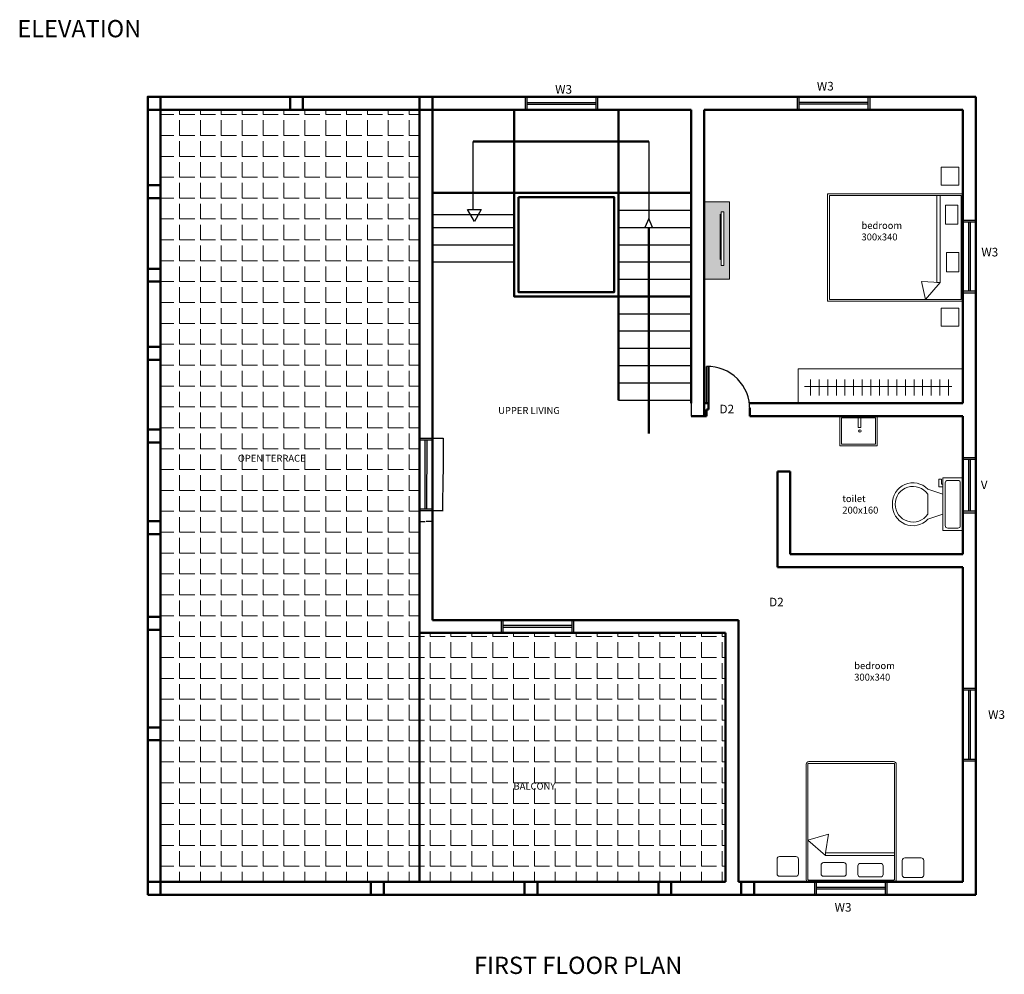
# Model space of a CAD drawing. Units: metres. Extents: x 10365 to 12529, y 3661 to 6248.
# Tile 2 of 9: x 11388 to 12529, y 3687 to 4794. Entities that reach past the tile are written whole.
import ezdxf

# ---------------------------------------------------------------- set-up
doc = ezdxf.new("R2010")
doc.units = ezdxf.units.M
doc.header["$MEASUREMENT"] = 0
for name, color, linetype, lineweight in [('A-ANNO-DIMS', 2, 'Continuous', 18), ('A-ANNO-TEXT', 7, 'Continuous', 18), ('A-AREA-IDEN', 7, 'Continuous', 18), ('A-DOOR', 4, 'Continuous', 25), ('A-FLOR-FIXT', 8, 'Continuous', 18), ('A-FLOR-PATT', 252, 'Continuous', 13), ('A-FLOR-STRS', 3, 'Continuous', 25), ('A-FURN', 30, 'Continuous', 18), ('A-GLAZ', 4, 'Continuous', 25), ('A-WALL', 7, 'Continuous', 50)]:
    doc.layers.add(name, color=color, linetype=linetype, lineweight=lineweight)
doc.styles.get("Standard").update_dxf_attribs({"font": 'arial.ttf'})
doc.dimstyles.get("Standard").update_dxf_attribs({"dimtxt": 0.18, "dimasz": 0.18, "dimexe": 0.18, "dimexo": 0.0625, "dimgap": 0.09, "dimtad": 0, "dimtih": 1, "dimtoh": 1, "dimdec": 0, "dimzin": 0, "dimdsep": 46, "dimtxsty": 'Standard', "dimcen": 0.09, "dimadec": 0, "dimazin": 0, "dimtfac": 1, "dimtdec": 0, "dimtofl": 0, "dimtmove": 0, "dimatfit": 3, "dimfxl": 1, "dimtolj": 1, "dimtzin": 0, "dimarcsym": 0})

# ---------------------------------------------------------------- blocks, each defined once
blk = doc.blocks.new('*U2')
for p, q in [((9.5, -6), (9.5, -2)), ((-10, -8.5), (-8, -8.5)), ((-10, -9.5), (-10, -8.5)), ((-7, -9.5), (-10, -9.5)), ((-8, -8.5), (-8, -8)), ((-7, -8), (-7, -9.5)), ((-4, -8), (-6, -14)), ((4, -8), (6, -14)), ((4, -14), (-4, -14))]:
    blk.add_line(p, q)
blk.add_lwpolyline([(10.5, -8), (10.5, 0), (-10.5, 0), (-10.5, -8)], close=True)
for points in [[(-9.5, -2), (-9.5, -6)], [(8.5, -1), (-8.5, -1)], [(-8.5, -7), (8.5, -7)]]:
    blk.add_lwpolyline(points)
for centre, radius, start, end in [((-8.625, -1.875), 0.8839, 81.8699, 188.1301), ((8.625, -1.875), 0.8839, 351.8699, 98.1301), ((-8.625, -6.125), 0.8839, 171.869898, 278.1301), ((8.625, -6.125), 0.8839, 261.8699, 8.1301), ((-0.4772, -19.9188), 8.0953, 133.01722, 273.38), ((0.0374, -19.8731), 7.127, 124.50543, 269.7), ((-0.0373, -19.8731), 7.127, 270.3, 55.4946), ((0.4773, -19.9188), 8.0953, 266.62, 46.9828)]:
    blk.add_arc(centre, radius, start, end)
blk = doc.blocks.new('DOOR-D2')
blk.add_line((0, 7.5), (0, 50))
blk.add_arc((1, 1), 49, 358.8309, 91.1691)
blk = doc.blocks.new('WIN-800')
for p, q in [((0, 0), (0, 15)), ((2, 0), (2, 15)), ((82, 0), (82, 15)), ((84, 0), (84, 15)), ((2, 8.5), (82, 8.5)), ((2, 6.5), (82, 6.5))]:
    blk.add_line(p, q)
blk = doc.blocks.new('VENT-600')
for p, q in [((0, 64), (15, 64)), ((0, 62), (15, 62)), ((6.5, 62), (6.5, 2)), ((8.5, 62), (8.5, 2)), ((8.5, 62), (8.5, 2)), ((0, 2), (15, 2)), ((0, 0), (15, 0))]:
    blk.add_line(p, q)
blk = doc.blocks.new('WIN-800-B')
for p, q in [((0, 84), (15, 84)), ((0, 82), (15, 82)), ((6.5, 82), (6.5, 2)), ((8.5, 82), (8.5, 2)), ((8.5, 82), (8.5, 2)), ((0, 2), (15, 2)), ((0, 0), (15, 0))]:
    blk.add_line(p, q)
blk = doc.blocks.new('*D19')
at = {"layer": 'A-ANNO-DIMS', "color": 0, "lineweight": -2, "transparency": 16777216}
for p, q in [((11866, 4308.7), (11878.7, 4308.6)), ((11878.6, 4308.4), (11878.4, 4266.8)), ((11878.3, 4224.8), (11878.4, 4266.4)), ((11865.7, 4224.7), (11878.5, 4224.6))]:
    blk.add_line(p, q, dxfattribs=at)
at = {"layer": 'A-ANNO-DIMS', "color": 0, "transparency": 16777216}
for points in [[(11878.5, 4308.4), (11878.6, 4308.4), (11878.6, 4308.6)], [(11878.3, 4224.8), (11878.3, 4224.8), (11878.3, 4224.6)]]:
    blk.add_solid(points, dxfattribs=at)
at = {"layer": 'Defpoints', "color": 0, "transparency": 16777216}
for p in [(11866, 4308.7), (11878.6, 4308.6), (11865.7, 4224.7)]:
    blk.add_point(p, dxfattribs=at)
at = {"layer": 'A-ANNO-DIMS', "color": 0, "transparency": 16777216, "insert": (11878.4, 4266.6), "char_height": 0.18, "attachment_point": 5}
blk.add_mtext('\\A1;WINDOW W3 84 TYP.', dxfattribs=at)
blk = doc.blocks.new('*D20')
at = {"layer": 'A-ANNO-DIMS', "color": 0, "lineweight": -2, "transparency": 16777216}
for p, q in [((11850.7, 4224.6), (11850.6, 4211.9)), ((11865.7, 4224.6), (11865.6, 4211.9)), ((11850.8, 4212.1), (11857.6, 4212.1)), ((11865.5, 4212.1), (11858.7, 4212.1))]:
    blk.add_line(p, q, dxfattribs=at)
at = {"layer": 'A-ANNO-DIMS', "color": 0, "transparency": 16777216}
for points in [[(11850.8, 4212.1), (11850.8, 4212.1), (11850.6, 4212.1)], [(11865.5, 4212.1), (11865.5, 4212), (11865.6, 4212.1)]]:
    blk.add_solid(points, dxfattribs=at)
at = {"layer": 'Defpoints', "color": 0, "transparency": 16777216}
for p in [(11850.7, 4224.7), (11865.7, 4224.7), (11865.6, 4212.1)]:
    blk.add_point(p, dxfattribs=at)
at = {"layer": 'A-ANNO-DIMS', "color": 0, "transparency": 16777216, "insert": (11858.1, 4212.1), "char_height": 0.18, "attachment_point": 5}
blk.add_mtext('\\A1;15 TYP.', dxfattribs=at)

msp = doc.modelspace()

# ---------------------------------------------------------------- hatches: boundary and pattern name
at = {"layer": 'A-FLOR-PATT'}
h = msp.add_hatch(dxfattribs=at)
h.set_pattern_fill('ANGLE', color=256, scale=88)
h.set_pattern_definition([(0, (2522.146, -930.819), (0, 24.2), [17.6, -6.6]), (90, (2522.146, -930.819), (-24.2, 1e-15), [17.6, -6.6])])
h.paths.add_polyline_path([(11551, 3794.2), (11876, 3794.2), (12206, 3794.2), (12206, 4082.8), (11851, 4082.8), (11851, 4689.2), (11551, 4689.2)])
at = {"layer": 'A-FURN'}
h = msp.add_hatch(color=256, dxfattribs=at)
h.dxf.hatch_style = 1
h.paths.add_polyline_path([(12210.4, 4582.5), (12181, 4582.5), (12181, 4492.7), (12210.4, 4492.7)])
h.paths.add_polyline_path([(12201, 4566.5), (12199.6, 4568.3), (12199.6, 4515.6), (12201, 4517.7)], flags=16)
h.paths.add_polyline_path([(12203.8, 4570.8), (12201, 4570.8), (12201, 4508.5), (12203.8, 4508.5)], flags=16)

# ---------------------------------------------------------------- linework, layer by layer
at = {"layer": 'A-FLOR-FIXT'}
for points in [[(12338.5, 4334.2), (12381.8, 4334.2), (12381.8, 4299.7), (12338.5, 4299.7)], [(12340.5, 4332.2), (12379.8, 4332.2), (12379.8, 4301.7), (12340.5, 4301.7)], [(12362.9, 4334.2), (12359.5, 4334.2), (12359.5, 4321.1), (12362.9, 4321.1)]]:
    msp.add_lwpolyline(points, close=True, dxfattribs=at)
msp.add_circle((12361.7, 4316.9), 1.49, dxfattribs=at)
at = {"layer": 'A-FLOR-STRS'}
for p, q in [((11913.4, 4573.4), (11913.4, 4652.4)), ((12116.8, 4652.4), (12116.8, 4563.3)), ((11866, 4567.8), (11960.8, 4567.8)), ((11906.9, 4573.4), (11922.7, 4573.4)), ((11914.8, 4559.7), (11906.9, 4573.4)), ((11922.7, 4573.4), (11914.8, 4559.7)), ((12081.8, 4572.8), (12166, 4572.8)), ((12116.8, 4563.3), (12112.5, 4552.8)), ((12121.3, 4552.8), (12116.8, 4563.3)), ((11866, 4552.8), (11960.8, 4552.8)), ((12081.8, 4552.8), (12166, 4552.8)), ((12116.8, 4552.8), (12121.3, 4552.8)), ((11866, 4532.8), (11960.8, 4532.8)), ((12081.8, 4532.8), (12166, 4532.8)), ((11866, 4512.8), (11960.8, 4512.8)), ((12081.8, 4512.8), (12166, 4512.8)), ((12081.8, 4492.8), (12166, 4492.8)), ((12081.8, 4452.8), (12166, 4452.8)), ((12081.8, 4432.8), (12166, 4432.8)), ((12081.8, 4412.8), (12166, 4412.8)), ((12081.8, 4392.8), (12166, 4392.8)), ((12081.8, 4372.8), (12166, 4372.8)), ((12081.8, 4352.8), (12166, 4352.8)), ((12166, 4349.2), (12166, 4334.2))]:
    msp.add_line(p, q, dxfattribs=at)
at = {"layer": 'A-FURN'}
for p, q in [((12201, 4566.5), (12199.6, 4568.3)), ((12199.6, 4568.3), (12199.6, 4515.6)), ((12199.6, 4515.6), (12201, 4517.7)), ((12437.8, 4469.2), (12433.1, 4490.1)), ((12433.1, 4490.1), (12454.8, 4489)), ((12454.8, 4489), (12437.8, 4469.2)), ((12290.1, 4349.2), (12290.1, 4388.8)), ((12290.1, 4388.8), (12481, 4388.8)), ((12304.4, 4376.6), (12304.4, 4358.2)), ((12314.4, 4376.6), (12314.4, 4358.2)), ((12324.4, 4376.6), (12324.4, 4358.2)), ((12334.4, 4376.6), (12334.4, 4358.2)), ((12344.4, 4376.6), (12344.4, 4358.2)), ((12354.4, 4376.6), (12354.4, 4358.2)), ((12364.4, 4376.6), (12364.4, 4358.2)), ((12374.4, 4376.6), (12374.4, 4358.2)), ((12384.4, 4376.6), (12384.4, 4358.2)), ((12394.4, 4376.6), (12394.4, 4358.2)), ((12404.4, 4376.6), (12404.4, 4358.2)), ((12414.4, 4376.6), (12414.4, 4358.2)), ((12424.4, 4376.6), (12424.4, 4358.2)), ((12434.4, 4376.6), (12434.4, 4358.2)), ((12444.4, 4376.6), (12444.4, 4358.2)), ((12454.4, 4376.6), (12454.4, 4358.2)), ((12464.4, 4376.6), (12464.4, 4358.2)), ((12297.4, 4368.4), (12468.3, 4368.4)), ((12301.4, 3842.6), (12325.3, 3849.8)), ((12325.3, 3849.8), (12321.7, 3828.1)), ((12321.7, 3825), (12301.4, 3842.6))]:
    msp.add_line(p, q, dxfattribs=at)
for points in [[(12455.7, 4622.7), (12476.2, 4622.7), (12476.2, 4601.8), (12455.7, 4601.8)], [(12481, 4591.7), (12324.3, 4591.7), (12324.3, 4467.2), (12481, 4467.2)], [(12479, 4589.7), (12326.3, 4589.7), (12326.3, 4469.2), (12479, 4469.2)], [(12451, 4589.7), (12454.8, 4589.7), (12454.8, 4489), (12451, 4489)], [(12181, 4582.5), (12210.4, 4582.5), (12210.4, 4492.7), (12181, 4492.7)], [(12461, 4578.7), (12475.4, 4578.7), (12475.4, 4556.5), (12461, 4556.5)], [(12201, 4570.8), (12203.8, 4570.8), (12203.8, 4508.5), (12201, 4508.5)], [(12462, 4523.7), (12476.4, 4523.7), (12476.4, 4501.5), (12462, 4501.5)], [(12455.9, 4459.1), (12476.4, 4459.1), (12476.4, 4438.2), (12455.9, 4438.2)], [(12401.8, 3825), (12401.8, 3825), (12321.7, 3825), (12321.7, 3825), (12321.7, 3828.1), (12321.7, 3828.1), (12401.8, 3828.1), (12401.8, 3828.1)]]:
    msp.add_lwpolyline(points, close=True, dxfattribs=at)
for points in [[(12403.8, 3797.2, -0.414214), (12400.8, 3794.2), (12302.4, 3794.2, -0.414214), (12299.4, 3797.2), (12299.4, 3930.7, -0.414214), (12302.4, 3933.7), (12400.8, 3933.7, -0.414214), (12403.8, 3930.7)], [(12401.8, 3797.2, -0.414214), (12400.8, 3796.2), (12302.4, 3796.2, -0.414214), (12301.4, 3797.2), (12301.4, 3930.7, -0.414214), (12302.4, 3931.7), (12400.8, 3931.7, -0.414214), (12401.8, 3930.7)], [(12265.6, 3820.7, -0.414214), (12268.6, 3823.7), (12287.5, 3823.7, -0.414214), (12290.5, 3820.7), (12290.5, 3803.8, -0.414214), (12287.5, 3800.8), (12268.6, 3800.8, -0.414214), (12265.6, 3803.8)], [(12316.6, 3813.6, -0.414214), (12319.6, 3816.6), (12342.9, 3816.6, -0.414214), (12345.9, 3813.6), (12345.9, 3803.8, -0.414214), (12342.9, 3800.8), (12319.6, 3800.8, -0.414214), (12316.6, 3803.8)], [(12359.3, 3812.8, -0.414214), (12362.3, 3815.8), (12385.6, 3815.8, -0.414214), (12388.6, 3812.8), (12388.6, 3803, -0.414214), (12385.6, 3800), (12362.3, 3800, -0.414214), (12359.3, 3803)], [(12410.8, 3819.1, -0.414214), (12413.8, 3822.1), (12432.7, 3822.1, -0.414214), (12435.7, 3819.1), (12435.7, 3802.2, -0.414214), (12432.7, 3799.2), (12413.8, 3799.2, -0.414214), (12410.8, 3802.2)]]:
    msp.add_lwpolyline(points, format="xyb", close=True, dxfattribs=at)
at = {"layer": 'A-WALL'}
for p, q in [((11786.8, 4704.2), (11536, 4704.2)), ((11536, 4704.2), (11536, 4349.2)), ((11536, 4704.2), (11851, 4704.2)), ((11851, 4704.2), (12496, 4704.2)), ((11866, 4704.2), (12166, 4704.2)), ((12496, 4704.2), (12496, 3779.2)), ((11851, 4689.2), (11551, 4689.2)), ((11551, 4689.2), (11551, 3794.2)), ((11851, 4082.8), (11851, 4689.2)), ((11866, 4334.2), (11866, 4689.2)), ((11866, 4689.2), (12166, 4689.2)), ((11960.8, 4689.2), (11960.8, 4472.8)), ((12081.8, 4689.2), (12081.8, 4352.8)), ((12166, 4689.2), (12166, 4349.2)), ((12181, 4689.2), (12181, 4349.2)), ((12181, 4689.2), (12481, 4689.2)), ((12481, 4689.2), (12481, 4349.2)), ((11913.4, 4652.4), (12116.8, 4652.4)), ((11866, 4592.8), (12166, 4592.8)), ((12116.8, 4552.8), (12116.8, 4314)), ((11866, 4512.8), (11866, 4097.8)), ((11960.8, 4472.8), (12166, 4472.8)), ((12186, 4341.7), (12186, 4391.7)), ((11536, 4349.2), (11536, 4334.2)), ((11851, 4349.2), (11851, 4334.2)), ((12186, 4349.2), (12181, 4349.2)), ((12181, 4349.2), (12181, 4334.2)), ((12481, 4349.2), (12233.5, 4349.2)), ((12184, 4341.7), (12184, 4334.2)), ((12186, 4341.7), (12184, 4341.7)), ((12234, 4343.7), (12234, 4334.2)), ((11536, 4334.2), (11536, 4004.2)), ((11551, 4334.2), (11551, 4004.2)), ((12184, 4334.2), (12166, 4334.2)), ((12481, 4334.2), (12234, 4334.2)), ((12481, 4334.2), (12481, 4174.2)), ((12496, 4334.2), (12496, 3779.2)), ((12266, 4159.2), (12266, 4270.1)), ((12281, 4270.1), (12266, 4270.1)), ((12281, 4174.2), (12281, 4270.1)), ((12481, 4174.2), (12281, 4174.2)), ((12481, 4159.2), (12266, 4159.2)), ((12481, 4159.2), (12481, 3794.2)), ((12496, 4159.2), (12496, 3779.2)), ((12221, 4097.8), (11866, 4097.8)), ((12221, 3794.2), (12221, 4097.8)), ((12206, 4082.8), (11851, 4082.8)), ((11851, 4082.8), (11851, 3794.2)), ((12206, 3794.2), (12206, 4082.8)), ((11536, 4004.2), (11536, 3989.2)), ((11536, 3989.2), (11536, 3779.2)), ((11551, 3989.2), (11551, 3794.2)), ((11551, 3794.2), (11876, 3794.2)), ((11876, 3794.2), (12206, 3794.2)), ((12221, 3794.2), (12481, 3794.2)), ((11536, 3779.2), (11876, 3779.2)), ((11536, 3779.2), (12496, 3779.2)), ((11876, 3779.2), (12206, 3779.2))]:
    msp.add_line(p, q, dxfattribs=at)
for points in [[(11536, 4689.2), (11536, 4689.2), (11551, 4689.2), (11551, 4689.2), (11551, 4704.2), (11551, 4704.2), (11536, 4704.2), (11536, 4704.2)], [(11701, 4689.2), (11701, 4689.2), (11716, 4689.2), (11716, 4689.2), (11716, 4704.2), (11716, 4704.2), (11701, 4704.2), (11701, 4704.2)], [(11851, 4689.2), (11851, 4689.2), (11866, 4689.2), (11866, 4689.2), (11866, 4704.2), (11866, 4704.2), (11851, 4704.2), (11851, 4704.2)], [(11536, 4586.7), (11536, 4586.7), (11551, 4586.7), (11551, 4586.7), (11551, 4601.7), (11551, 4601.7), (11536, 4601.7), (11536, 4601.7)], [(11960.8, 4592.8), (12081.8, 4592.8), (12081.8, 4472.8), (11960.8, 4472.8)], [(11965.8, 4587.8), (12076.8, 4587.8), (12076.8, 4477.8), (11965.8, 4477.8)], [(11536, 4490), (11536, 4490), (11551, 4490), (11551, 4490), (11551, 4505), (11551, 4505), (11536, 4505), (11536, 4505)], [(11536, 4399.5), (11536, 4399.5), (11551, 4399.5), (11551, 4399.5), (11551, 4414.5), (11551, 4414.5), (11536, 4414.5), (11536, 4414.5)], [(11536, 4303.7), (11536, 4303.7), (11551, 4303.7), (11551, 4303.7), (11551, 4318.7), (11551, 4318.7), (11536, 4318.7), (11536, 4318.7)], [(11536, 4197.3), (11536, 4197.3), (11551, 4197.3), (11551, 4197.3), (11551, 4212.3), (11551, 4212.3), (11536, 4212.3), (11536, 4212.3)], [(11536, 4086.4), (11536, 4086.4), (11551, 4086.4), (11551, 4086.4), (11551, 4101.4), (11551, 4101.4), (11536, 4101.4), (11536, 4101.4)], [(11536, 3958.4), (11536, 3958.4), (11551, 3958.4), (11551, 3958.4), (11551, 3973.4), (11551, 3973.4), (11536, 3973.4), (11536, 3973.4)], [(11536, 3779.2), (11536, 3779.2), (11551, 3779.2), (11551, 3779.2), (11551, 3794.2), (11551, 3794.2), (11536, 3794.2), (11536, 3794.2)], [(11794.7, 3779.2), (11794.7, 3779.2), (11809.7, 3779.2), (11809.7, 3779.2), (11809.7, 3794.2), (11809.7, 3794.2), (11794.7, 3794.2), (11794.7, 3794.2)], [(11972.9, 3779.2), (11972.9, 3779.2), (11987.9, 3779.2), (11987.9, 3779.2), (11987.9, 3794.2), (11987.9, 3794.2), (11972.9, 3794.2), (11972.9, 3794.2)], [(12128, 3779.2), (12128, 3779.2), (12143, 3779.2), (12143, 3779.2), (12143, 3794.2), (12143, 3794.2), (12128, 3794.2), (12128, 3794.2)], [(12224, 3779.2), (12224, 3779.2), (12239, 3779.2), (12239, 3779.2), (12239, 3794.2), (12239, 3794.2), (12224, 3794.2), (12224, 3794.2)]]:
    msp.add_lwpolyline(points, close=True, dxfattribs=at)
msp.add_lwpolyline([(11960.8, 4472.8), (11960.8, 4592.8), (12081.8, 4592.8), (12081.8, 4432.8)], dxfattribs=at)

# ---------------------------------------------------------------- block references
at = {"layer": 'A-DOOR'}
msp.add_blockref('DOOR-D2', (12184, 4341.7), dxfattribs=at)
at = {"layer": 'A-FLOR-FIXT', "xscale": 2.907913259437767, "yscale": 2.907913259437767, "zscale": 2.907913259437767, "rotation": 270}
msp.add_blockref('*U2', (12481, 4232), dxfattribs=at)
at = {"layer": 'A-GLAZ'}
for name, p in [('WIN-800', (11974, 4689.2)), ('VENT-600', (12481, 4222.2)), ('WIN-800-B', (12481, 3934.7))]:
    msp.add_blockref(name, p, dxfattribs=at)
for name, p, rotation in [('WIN-800', (12373, 4704.2), 180), ('WIN-800', (12481, 4561.2), 270.0000000000017), ('WIN-800-B', (11850.7, 4224.7), 359.8112505414526), ('WIN-800', (12029.7, 4097.8), 180), ('WIN-800', (12393, 3794.2), 180)]:
    msp.add_blockref(name, p, dxfattribs=dict(at, rotation=rotation))

# ---------------------------------------------------------------- texts
at = {"layer": 'A-ANNO-TEXT', "attachment_point": 1}
for s, width, insert, char_height in [('ELEVATION', 412.275, (11384.9, 4793.2), 20), ('W3', 63.407, (12008.4, 4717.8), 10), ('W3', 63.407, (12311.8, 4721.5), 10), ('W3', 63.407, (12502.5, 4529.2), 10), ('D2', 63.407, (12198.9, 4347.3), 10), ('V', 63.407, (12501.8, 4259.5), 10), ('D2', 63.407, (12256.4, 4123.6), 10), ('W3', 63.407, (12510.3, 3993.2), 10), ('W3', 63.407, (12332.4, 3769.8), 10), ('FIRST FLOOR PLAN', 412.275, (11914.4, 3707.6), 20)]:
    msp.add_mtext_dynamic_manual_height_columns(s, width=width, gutter_width=1, heights=[0], dxfattribs=dict(at, insert=insert, char_height=char_height))
at = {"layer": 'A-AREA-IDEN', "char_height": 8, "attachment_point": 1}
for s, insert in [('bedroom\\P300x340', (12363.5, 4559.1)), ('UPPER LIVING', (11942.3, 4344.6)), ('OPEN TERRACE', (11640.5, 4289.3)), ('toilet\\P200x160', (12341.3, 4242.5)), ('bedroom\\P300x340', (12355.1, 4048.9)), ('BALCONY', (11960.1, 3909.2))]:
    msp.add_mtext_dynamic_manual_height_columns(s, width=106.401, gutter_width=1, heights=[0], dxfattribs=dict(at, insert=insert))

# ---------------------------------------------------------------- dimensions: what is measured, and where the dimension line sits
at = {"layer": 'A-ANNO-DIMS'}
for base, p1, p2, angle, text, picture, middle in [((11878.6, 4308.6), (11865.7, 4224.7), (11866, 4308.7), 89.8113, 'WINDOW W3 <> TYP.', '*D19', (11878.4, 4266.6)), ((11865.6, 4212.1), (11850.7, 4224.7), (11865.7, 4224.7), 359.8113, '<> TYP.', '*D20', (11858.1, 4212.1))]:
    dim = msp.add_linear_dim(base=base, p1=p1, p2=p2, angle=angle, text=text, dimstyle='Standard', override={"dimdec": 0, "dimrnd": 0, "dimzin": 0, "dimlunit": 2}, dxfattribs=at)
    dim.commit()
    dim.dimension.update_dxf_attribs({"geometry": picture, "text_midpoint": middle})

doc.saveas('drawing.dxf')
